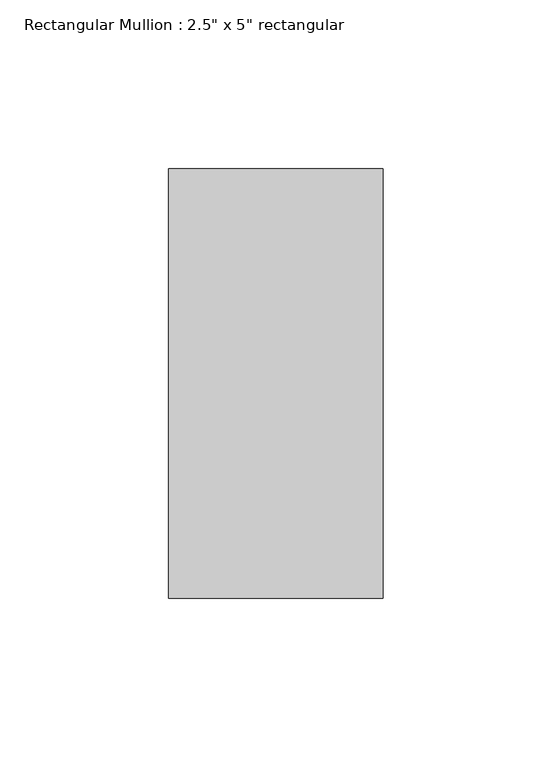
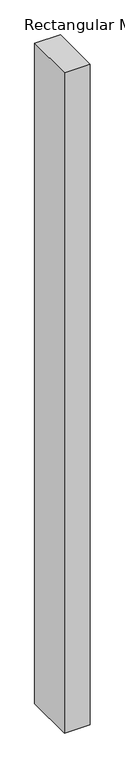
"""IFC4 building model written with IfcOpenShell, lengths in millimetres: member geometry."""

from ifc_helpers import new_model, si_unit, frame, origin, place, context, project, spatial, polyline, outline, extrude, source, transform, mapped, element, save


def member_fceb641e(model_context):
    return source(origin(), model_context, "Body", "SweptSolid", [
        extrude(outline(polyline([(31.75, 63.5), (31.75, -63.5), (-31.75, -63.5), (-31.75, 63.5), (31.75, 63.5)])), frame((0.0, 0.0, -1725.9311114), z_axis=(0.0, 0.0, 1.0), x_axis=(1.0, 0.0, 0.0)), (0.0, 0.0, 1.0), 1725.9311114),
    ])


if __name__ == "__main__":
    model = new_model("IFC4")
    model_context = context("Model", 3, world=origin())
    ifc_project = project(units=[si_unit("LENGTHUNIT", "METRE", prefix="MILLI")], contexts=[model_context])
    site = spatial("IfcSite", under=ifc_project)
    building = spatial("IfcBuilding", under=site)
    placement = place(None, origin())
    member_shape = member_fceb641e(model_context)
    element("IfcMember", 1, ObjectType="Rectangular Mullion : 2.5\" x 5\" rectangular", at=placement, inside=building, context=model_context, shape_type="MappedRepresentation", body=[
        mapped(member_shape, transform((0.0, 0.0, 0.0), x_axis=(1.0, 0.0, 0.0), y_axis=(0.0, 1.0, 0.0), z_axis=(0.0, 0.0, 1.0))),
    ])
    save(model, "model.ifc")

# Revit data of these elements
# Type "Rectangular Mullion : 2.5\" x 5\" rectangular"
#   built-in parameter 1007304 = 0.416667 (stored number, unit not read)
#   built-in parameter 1007301 = 0.104167 (stored number, unit not read)
#   built-in parameter 1007300 = 0.104167 (stored number, unit not read)
# Element 1 (IfcMember, "Rectangular Mullion : 2.5\" x 5\" rectangular")
#   Materials on its faces: "Aluminum"
# Materials
#   "Aluminum": class "Metal", colour RGB 247 247 247, transparency 0, Description = "Aluminum 6061", Cost = 0
